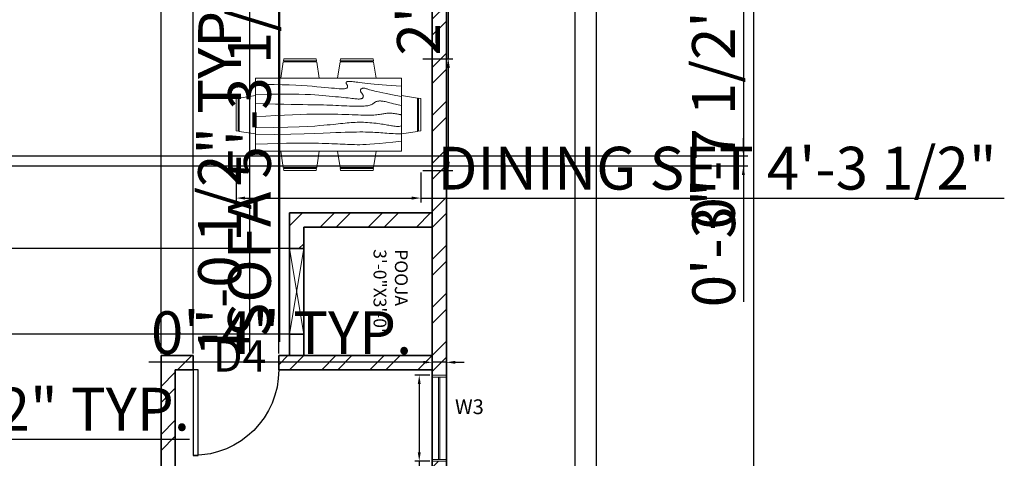
# Model space of a CAD drawing. Units: inches. Extents: x 2242 to 2870, y 1782 to 2635.
# Tile 4 of 7: x 2594 to 2870, y 2020 to 2143. Entities that reach past the tile are written whole.
import ezdxf

# ---------------------------------------------------------------- set-up
doc = ezdxf.new("R2010")
doc.units = ezdxf.units.IN
for name, color, linetype, lineweight in [('A-ANNO-DIMS', 7, 'Continuous', 18), ('A-ANNO-TEXT', 1, 'Continuous', 18), ('A-AREA-IDEN', 1, 'Continuous', 25), ('A-WALL-PATT', 253, 'Continuous', 13), ('C-PROP', 7, 'Continuous', 30), ('doors', 5, 'Continuous', 25), ('furniture', 9, 'Continuous', 18), ('walls', 7, 'Continuous', 35), ('windows', 72, 'Continuous', 18)]:
    doc.layers.add(name, color=color, linetype=linetype, lineweight=lineweight)
doc.styles.get("Standard").update_dxf_attribs({"font": 'arial.ttf'})
doc.dimstyles.new('ISO-25', dxfattribs={"dimtxt": 12, "dimasz": 2.5, "dimexe": 1.25, "dimexo": 0.625, "dimtad": 1, "dimlunit": 4, "dimtxsty": 'Standard', "dimcen": 2.5, "dimadec": 0, "dimazin": 0, "dimtfac": 1, "dimtmove": 0, "dimatfit": 3, "dimfxl": 1, "dimarcsym": 0})

# ---------------------------------------------------------------- blocks, each defined once
blk = doc.blocks.new('*U2')
for p, q in [((0, 0), (0, -5)), ((30, 0), (30, -5))]:
    blk.add_line(p, q)
blk.add_lwpolyline([(0, 0), (0, 30), (1.75, 30), (1.75, 0)], close=True)
blk.add_arc((0, 0), 30, 0, 90)
blk = doc.blocks.new('Dining Set - 36 x 72 in.')
for p, q in [((-22.2343, 26.00059), (-23.4847, 17.99762)), ((-22.2304, 26), (-5.7608, 26)), ((-22, 27.5), (-22.1562, 26.50042)), ((-5.8416, 26.5), (-22.1534, 26.5)), ((-22, 27.5), (-6, 27.5)), ((-5.8437, 26.49966), (-6, 27.5)), ((-4.5152, 17.99762), (-5.7655, 25.99926)), ((5.7657, 26.00059), (4.5153, 17.99762)), ((5.7696, 26), (22.2392, 26)), ((6, 27.5), (5.8438, 26.50042)), ((22.1584, 26.5), (5.8466, 26.5)), ((6, 27.5), (22, 27.5)), ((22.1563, 26.49966), (22, 27.5)), ((23.4848, 17.99762), (22.2345, 25.99926)), ((36, 18), (-36, 18)), ((-36, 18), (-36, -18)), ((36, -18), (36, 18)), ((-45.5, 8), (-44.5004, 8.15617)), ((-45.5, 8), (-45.5, -8)), ((-44.5, -8.15843), (-44.5, 8.15338)), ((-44.0006, 8.23428), (-35.9976, 9.48474)), ((-44, 8.23041), (-44, -8.23915)), ((44.0006, 8.23428), (35.9976, 9.48474)), ((44, 8.23041), (44, -8.23915)), ((44.5, -8.15843), (44.5, 8.15338)), ((45.5, 8), (44.5005, 8.15617)), ((45.5, 8), (45.5, -8)), ((-44.4997, -8.15631), (-45.5, -8)), ((-35.9976, -9.48476), (-43.9993, -8.2345)), ((35.9976, -9.48476), (43.9993, -8.2345)), ((44.4997, -8.15631), (45.5, -8)), ((-36, -18), (36, -18)), ((-22.2343, -26.0006), (-23.4847, -17.99762)), ((-4.5152, -17.99762), (-5.7655, -25.99928)), ((5.7657, -26.0006), (4.5153, -17.99762)), ((23.4848, -17.99762), (22.2345, -25.99928)), ((-22.2304, -26), (-5.7608, -26)), ((-22, -27.5), (-22.1562, -26.50044)), ((-5.8416, -26.5), (-22.1534, -26.5)), ((-22, -27.5), (-6, -27.5)), ((-5.8437, -26.49967), (-6, -27.5)), ((5.7696, -26), (22.2392, -26)), ((6, -27.5), (5.8438, -26.50044)), ((22.1584, -26.5), (5.8466, -26.5)), ((6, -27.5), (22, -27.5)), ((22.1563, -26.49967), (22, -27.5))]:
    blk.add_line(p, q)
for points in [[(-36, 15), (-31.1772, 14.97754), (-26.8079, 14.91406), (-22.8538, 14.81543), (-19.276, 14.6875), (-16.0362, 14.53613), (-13.0957, 14.36718), (-10.4159, 14.18652), (-7.9583, 14), (-5.6904, 13.81315), (-3.6035, 13.63021), (-1.6954, 13.45508), (0.0365, 13.29166), (1.5945, 13.14388), (2.9811, 13.01562), (4.1988, 12.9108), (5.25, 12.83333), (6.1393, 12.78613), (6.8802, 12.76823), (7.4883, 12.77767), (7.9792, 12.8125), (8.3685, 12.87077), (8.6719, 12.95052), (8.9049, 13.0498), (9.0833, 13.16666), (9.2205, 13.29899), (9.3216, 13.44401), (9.3895, 13.59879), (9.4271, 13.76041), (9.4373, 13.92594), (9.4232, 14.09245), (9.3875, 14.257), (9.3333, 14.41666), (9.2638, 14.56917), (9.1836, 14.71484), (9.0975, 14.85465), (9.0104, 14.98958), (8.9272, 15.1206), (8.8529, 15.2487), (8.7922, 15.37483), (8.75, 15.5), (8.7305, 15.62467), (8.7344, 15.74739), (8.7617, 15.86621), (8.8125, 15.97916), (8.8867, 16.08431), (8.9844, 16.17968), (9.1055, 16.26334), (9.25, 16.33333), (9.4189, 16.38802), (9.6172, 16.42708), (9.8506, 16.45052), (10.125, 16.45833), (10.4463, 16.45052), (10.8203, 16.42708), (11.2529, 16.38802), (11.75, 16.33333), (12.3184, 16.26318), (12.9694, 16.17838), (13.7151, 16.07991), (14.5677, 15.96875), (15.5395, 15.84586), (16.6426, 15.71224), (17.8893, 15.56884), (19.2917, 15.41666), (20.859, 15.25667), (22.5879, 15.08984), (24.4721, 14.91715), (26.5052, 14.73958), (28.6809, 14.5581), (30.9929, 14.3737), (33.4347, 14.18733), (36, 14)], [(-36, 10), (-28.9766, 10.14274), (-23.1725, 10.20442), (-18.4241, 10.19775), (-14.5677, 10.13541), (-11.4399, 10.03011), (-8.877, 9.89453), (-6.7154, 9.74137), (-4.7917, 9.58333), (-2.9698, 9.43082), (-1.2246, 9.28515), (0.4415, 9.14534), (2.026, 9.01041), (3.5266, 8.87939), (4.9408, 8.7513), (6.266, 8.62516), (7.5, 8.5), (8.6411, 8.37549), (9.6914, 8.2539), (10.6538, 8.13818), (11.5312, 8.03125), (12.3267, 7.93603), (13.043, 7.85547), (13.6831, 7.79248), (14.25, 7.75), (14.7471, 7.7303), (15.1797, 7.73307), (15.5537, 7.75732), (15.875, 7.80208), (16.1494, 7.86637), (16.3828, 7.94922), (16.5811, 8.04964), (16.75, 8.16666), (16.8944, 8.29915), (17.0143, 8.44531), (17.1089, 8.60319), (17.1771, 8.77083), (17.218, 8.94629), (17.2305, 9.1276), (17.2137, 9.31282), (17.1667, 9.5), (17.0895, 9.6875), (16.987, 9.875), (16.8649, 10.0625), (16.7292, 10.25), (16.5856, 10.4375), (16.4401, 10.625), (16.2985, 10.8125), (16.1667, 11), (16.05, 11.18733), (15.9518, 11.3737), (15.8752, 11.5581), (15.8229, 11.73958), (15.798, 11.91715), (15.8034, 12.08984), (15.842, 12.25667), (15.9167, 12.41666), (16.0295, 12.56836), (16.1784, 12.70833), (16.3605, 12.83268), (16.5729, 12.9375), (16.8127, 13.01888), (17.0768, 13.07291), (17.3625, 13.0957), (17.6667, 13.08333), (17.9894, 13.03312), (18.3418, 12.94726), (18.7382, 12.82918), (19.1927, 12.68229), (19.7195, 12.51001), (20.3327, 12.31575), (21.0465, 12.10294), (21.875, 11.875), (22.8357, 11.63354), (23.959, 11.37304), (25.2786, 11.08618), (26.8282, 10.76562), (28.6414, 10.40405), (30.752, 9.99414), (33.1936, 9.52856), (36, 9)], [(-36, 5.5), (-30.7157, 5.3348), (-26.069, 5.20963), (-21.9946, 5.11767), (-18.4271, 5.05208), (-15.3009, 5.00602), (-12.5508, 4.97265), (-10.1112, 4.94515), (-7.9167, 4.91666), (-5.909, 4.88167), (-4.0586, 4.83984), (-2.3429, 4.79215), (-0.7396, 4.73958), (0.7739, 4.6831), (2.22, 4.6237), (3.6213, 4.56233), (5, 4.5), (6.373, 4.43782), (7.7344, 4.3776), (9.0723, 4.32129), (10.375, 4.27083), (11.6309, 4.22819), (12.8281, 4.19531), (13.9551, 4.17415), (15, 4.16666), (15.954, 4.17448), (16.819, 4.19791), (17.6001, 4.23698), (18.3021, 4.29166), (18.9299, 4.36198), (19.4883, 4.44791), (19.9823, 4.54948), (20.4167, 4.66666), (20.7969, 4.79899), (21.1302, 4.94401), (21.4245, 5.09879), (21.6875, 5.26041), (21.9271, 5.42594), (22.1511, 5.59245), (22.3672, 5.757), (22.5834, 5.91666), (22.8065, 6.06868), (23.0404, 6.21093), (23.2879, 6.34147), (23.5521, 6.45833), (23.8358, 6.55957), (24.142, 6.64323), (24.4735, 6.70735), (24.8334, 6.75), (25.2235, 6.76969), (25.642, 6.76692), (26.0858, 6.74267), (26.5521, 6.69791), (27.0379, 6.63362), (27.5404, 6.55078), (28.0565, 6.45036), (28.5834, 6.33333), (29.1242, 6.19987), (29.7071, 6.04687), (30.3661, 5.87044), (31.1354, 5.66666), (32.0493, 5.43164), (33.142, 5.16146), (34.4475, 4.85221), (36, 4.5)], [(-36, -1), (-30.7915, -0.6591), (-26.0195, -0.38216), (-21.6519, -0.16284), (-17.6563, 0.00521), (-14.0005, 0.12833), (-10.6523, 0.21289), (-7.5796, 0.26522), (-4.75, 0.29166), (-2.134, 0.29793), (0.2878, 0.28711), (2.5317, 0.26163), (4.6146, 0.22396), (6.5529, 0.17651), (8.3633, 0.12174), (10.0623, 0.06209), (11.6667, 0), (13.1899, -0.06201), (14.6341, -0.1211), (15.9982, -0.17432), (17.2813, -0.21875), (18.4823, -0.25147), (19.6003, -0.26953), (20.6343, -0.27002), (21.5834, -0.25), (22.4481, -0.20768), (23.2357, -0.14584), (23.9549, -0.06836), (24.6146, 0.02083), (25.2235, 0.11784), (25.7904, 0.21875), (26.3241, 0.31966), (26.8334, 0.41666), (27.3265, 0.50618), (27.8099, 0.58593), (28.2894, 0.65397), (28.7709, 0.70833), (29.2601, 0.74707), (29.763, 0.76823), (30.2855, 0.76985), (30.8334, 0.75), (31.4088, 0.70784), (31.9994, 0.64713), (32.589, 0.57275), (33.1615, 0.48958), (33.7008, 0.4025), (34.1908, 0.3164), (34.6153, 0.23616), (34.9584, 0.16666), (35.2099, 0.11165), (35.3848, 0.07031), (35.504, 0.04069), (35.5886, 0.02083), (35.6594, 0.00879), (35.7377, 0.0026), (35.8442, 0.00032), (36, 0)], [(-36, -6.5), (-27.1843, -6.31267), (-20.084, -6.1263), (-14.469, -5.9419), (-10.1094, -5.76042), (-6.7752, -5.58285), (-4.2363, -5.41016), (-2.2629, -5.24333), (-0.625, -5.08334), (0.8708, -4.93099), (2.2715, -4.78646), (3.5872, -4.64974), (4.8281, -4.52084), (6.0046, -4.39974), (7.127, -4.28646), (8.2053, -4.18099), (9.25, -4.08334), (10.2705, -3.99382), (11.2734, -3.91407), (12.2647, -3.84603), (13.25, -3.79167), (14.2354, -3.75293), (15.2266, -3.73177), (16.2295, -3.73015), (17.25, -3.75), (18.2912, -3.79248), (19.3451, -3.85547), (20.4009, -3.93604), (21.4479, -4.03125), (22.4754, -4.13819), (23.4727, -4.25391), (24.4289, -4.37549), (25.3334, -4.5), (26.1785, -4.62492), (26.9694, -4.74935), (27.7145, -4.87281), (28.4219, -4.99479), (29.1, -5.11483), (29.7572, -5.23242), (30.4016, -5.34709), (31.0417, -5.45834), (31.6837, -5.56437), (32.3262, -5.65821), (32.9658, -5.73153), (33.599, -5.77604), (34.2224, -5.78345), (34.8327, -5.74545), (35.4264, -5.65373), (36, -5.5)], [(-36, -10), (-26.4022, -9.81299), (-18.4675, -9.62891), (-11.9839, -9.45069), (-6.7396, -9.28125), (-2.5226, -9.12354), (0.8789, -8.98047), (3.6769, -8.85498), (6.0833, -8.75), (8.2767, -8.66765), (10.3021, -8.60677), (12.1712, -8.56543), (13.8958, -8.54167), (15.4876, -8.53353), (16.9583, -8.53907), (18.3197, -8.55632), (19.5834, -8.58334), (20.7616, -8.61841), (21.8685, -8.66081), (22.9188, -8.71004), (23.9271, -8.76563), (24.9081, -8.82707), (25.8763, -8.89388), (26.8465, -8.96558), (27.8334, -9.04167), (28.8474, -9.12118), (29.8828, -9.20117), (30.93, -9.27824), (31.9792, -9.34896), (33.0205, -9.40991), (34.0443, -9.45768), (35.0407, -9.48885), (36, -9.5)], [(-36, -14.5), (-30.0881, -14.33513), (-25.0332, -14.21224), (-20.7312, -14.12647), (-17.0781, -14.07292), (-13.97, -14.04671), (-11.3027, -14.04297), (-8.9724, -14.05681), (-6.875, -14.08334), (-4.9224, -14.11833), (-3.0905, -14.16016), (-1.3709, -14.20785), (0.2448, -14.26042), (1.7647, -14.3169), (3.1973, -14.3763), (4.5507, -14.43767), (5.8333, -14.5), (7.0554, -14.5621), (8.235, -14.62175), (9.3922, -14.67652), (10.5469, -14.72396), (11.7192, -14.76164), (12.929, -14.78711), (14.1965, -14.79794), (15.5417, -14.79167), (16.9933, -14.76424), (18.6152, -14.70508), (20.4804, -14.60197), (22.6615, -14.44271), (25.2312, -14.21509), (28.2624, -13.9069), (31.8277, -13.50594), (36, -13)]]:
    blk.add_lwpolyline(points)
blk = doc.blocks.new('*D29')
at = {"layer": 'A-ANNO-DIMS', "color": 0, "lineweight": -2, "transparency": 16777216}
for p, q in [((2755.79, 2540.33), (2800.47, 2540.33)), ((2799.22, 2537.83), (2799.22, 1942.83)), ((2755.79, 1940.33), (2800.47, 1940.33))]:
    blk.add_line(p, q, dxfattribs=at)
at = {"layer": 'A-ANNO-DIMS', "color": 0, "transparency": 16777216}
for points in [[(2798.81, 2537.83), (2799.64, 2537.83), (2799.22, 2540.33)], [(2798.81, 1942.83), (2799.64, 1942.83), (2799.22, 1940.33)]]:
    blk.add_solid(points, dxfattribs=at)
at = {"layer": 'Defpoints', "color": 0, "transparency": 16777216}
for p in [(2755.16, 2540.33), (2755.16, 1940.33), (2799.22, 1940.33)]:
    blk.add_point(p, dxfattribs=at)
at = {"layer": 'A-ANNO-DIMS', "color": 0, "transparency": 16777216, "insert": (2792.47, 2240.33), "char_height": 12, "attachment_point": 5, "rotation": 90}
blk.add_mtext("50'", dxfattribs=at)
blk = doc.blocks.new('WIN-W3-24IN')
for p, q in [((0, 0), (0, 24.12)), ((0, 24.12), (4, 24.12)), ((0, 23.62), (4, 23.62)), ((1.8, 23.62), (1.8, 0.5)), ((2.2, 23.62), (2.2, 0.5)), ((4, 24.12), (4, 0)), ((4, 0.5), (0, 0.5)), ((4, 0), (0, 0))]:
    blk.add_line(p, q)
blk = doc.blocks.new('*D37')
at = {"layer": 'A-ANNO-DIMS', "color": 0, "lineweight": -2, "transparency": 16777216}
for p, q in [((2708.54, 2043.59), (2704.3, 2043.59)), ((2705.55, 2041.09), (2705.55, 2021.98)), ((2708.54, 2019.48), (2704.3, 2019.48)), ((2705.55, 2019.48), (2705.55, 1912.29))]:
    blk.add_line(p, q, dxfattribs=at)
at = {"layer": 'A-ANNO-DIMS', "color": 0, "transparency": 16777216}
for points in [[(2705.13, 2041.09), (2705.96, 2041.09), (2705.55, 2043.59)], [(2705.13, 2021.98), (2705.96, 2021.98), (2705.55, 2019.48)]]:
    blk.add_solid(points, dxfattribs=at)
at = {"layer": 'Defpoints', "color": 0, "transparency": 16777216}
for p in [(2709.16, 2043.59), (2705.55, 2019.48), (2709.16, 2019.48)]:
    blk.add_point(p, dxfattribs=at)
at = {"layer": 'A-ANNO-DIMS', "color": 0, "transparency": 16777216, "insert": (2698.79, 1964.63), "char_height": 12, "attachment_point": 5, "rotation": 90}
blk.add_mtext('W3 2\'-0" TYP.', dxfattribs=at)
blk = doc.blocks.new('*D38')
at = {"layer": 'A-ANNO-DIMS', "color": 0, "lineweight": -2, "transparency": 16777216}
for p, q in [((2709.16, 2044.22), (2709.16, 2048.46)), ((2713.16, 2044.22), (2713.16, 2048.46)), ((2706.66, 2047.21), (2629.77, 2047.21)), ((2713.16, 2047.21), (2709.16, 2047.21)), ((2715.66, 2047.21), (2718.16, 2047.21))]:
    blk.add_line(p, q, dxfattribs=at)
at = {"layer": 'A-ANNO-DIMS', "color": 0, "transparency": 16777216}
for points in [[(2706.66, 2047.63), (2706.66, 2046.79), (2709.16, 2047.21)], [(2715.66, 2047.63), (2715.66, 2046.79), (2713.16, 2047.21)]]:
    blk.add_solid(points, dxfattribs=at)
at = {"layer": 'Defpoints', "color": 0, "transparency": 16777216}
for p in [(2709.16, 2047.21), (2709.16, 2043.59), (2713.16, 2043.59)]:
    blk.add_point(p, dxfattribs=at)
at = {"layer": 'A-ANNO-DIMS', "color": 0, "transparency": 16777216, "insert": (2666.97, 2053.96), "char_height": 12, "attachment_point": 5}
blk.add_mtext('0\'-4" TYP.', dxfattribs=at)
blk = doc.blocks.new('*D42')
at = {"layer": 'A-ANNO-DIMS', "color": 0, "lineweight": -2, "transparency": 16777216}
for p, q in [((2522.93, 2020.21), (2522.93, 2026.94)), ((2537.42, 2020.21), (2537.42, 2026.94)), ((2525.43, 2025.69), (2534.92, 2025.69)), ((2537.42, 2025.69), (2641.15, 2025.69))]:
    blk.add_line(p, q, dxfattribs=at)
at = {"layer": 'A-ANNO-DIMS', "color": 0, "transparency": 16777216}
for points in [[(2525.43, 2026.11), (2525.43, 2025.28), (2522.93, 2025.69)], [(2534.92, 2026.11), (2534.92, 2025.28), (2537.42, 2025.69)]]:
    blk.add_solid(points, dxfattribs=at)
at = {"layer": 'Defpoints', "color": 0, "transparency": 16777216}
for p in [(2537.42, 2025.69), (2522.93, 2019.58), (2537.42, 2019.58)]:
    blk.add_point(p, dxfattribs=at)
at = {"layer": 'A-ANNO-DIMS', "color": 0, "transparency": 16777216, "insert": (2590.54, 2032.52), "char_height": 12, "attachment_point": 5}
blk.add_mtext('1\'-2 1/2" TYP.', dxfattribs=at)
blk = doc.blocks.new('*D44')
at = {"layer": 'A-ANNO-DIMS', "color": 0, "lineweight": -2, "transparency": 16777216}
for p, q in [((2659.56, 2164.94), (2656.71, 2164.94)), ((2657.96, 2162.44), (2657.96, 2155.17)), ((2659.56, 2152.67), (2656.71, 2152.67)), ((2657.96, 2152.67), (2657.96, 2048.94))]:
    blk.add_line(p, q, dxfattribs=at)
at = {"layer": 'A-ANNO-DIMS', "color": 0, "transparency": 16777216}
for points in [[(2657.54, 2162.44), (2658.38, 2162.44), (2657.96, 2164.94)], [(2657.54, 2155.17), (2658.38, 2155.17), (2657.96, 2152.67)]]:
    blk.add_solid(points, dxfattribs=at)
at = {"layer": 'Defpoints', "color": 0, "transparency": 16777216}
for p in [(2660.19, 2164.94), (2657.96, 2152.67), (2660.19, 2152.67)]:
    blk.add_point(p, dxfattribs=at)
at = {"layer": 'A-ANNO-DIMS', "color": 0, "transparency": 16777216, "insert": (2651.13, 2099.56), "char_height": 12, "attachment_point": 5, "rotation": 90}
blk.add_mtext('1\'-0 1/2" TYP.', dxfattribs=at)
blk = doc.blocks.new('*D51')
at = {"layer": 'A-ANNO-DIMS', "color": 0, "lineweight": -2, "transparency": 16777216}
for p, q in [((2654.22, 2100.4), (2654.22, 2092.02)), ((2705.95, 2100.4), (2705.95, 2092.02)), ((2656.72, 2093.27), (2703.45, 2093.27)), ((2705.95, 2093.27), (2869.55, 2093.27))]:
    blk.add_line(p, q, dxfattribs=at)
at = {"layer": 'A-ANNO-DIMS', "color": 0, "transparency": 16777216}
for points in [[(2656.72, 2093.69), (2656.72, 2092.85), (2654.22, 2093.27)], [(2703.45, 2093.69), (2703.45, 2092.85), (2705.95, 2093.27)]]:
    blk.add_solid(points, dxfattribs=at)
at = {"layer": 'Defpoints', "color": 0, "transparency": 16777216}
for p in [(2654.22, 2101.03), (2705.95, 2101.03), (2705.95, 2093.27)]:
    blk.add_point(p, dxfattribs=at)
at = {"layer": 'A-ANNO-DIMS', "color": 0, "transparency": 16777216, "insert": (2789, 2100.1), "char_height": 12, "attachment_point": 5}
blk.add_mtext('DINING SET 4\'-3 1/2"', dxfattribs=at)
blk = doc.blocks.new('*D52')
at = {"layer": 'A-ANNO-DIMS', "color": 0, "lineweight": -2, "transparency": 16777216}
for p, q in [((2713.71, 2132.29), (2713.71, 2196.1)), ((2706.57, 2132.29), (2714.96, 2132.29)), ((2713.71, 2103.53), (2713.71, 2129.79)), ((2706.57, 2101.03), (2714.96, 2101.03))]:
    blk.add_line(p, q, dxfattribs=at)
at = {"layer": 'A-ANNO-DIMS', "color": 0, "transparency": 16777216}
for points in [[(2713.29, 2129.79), (2714.12, 2129.79), (2713.71, 2132.29)], [(2713.29, 2103.53), (2714.12, 2103.53), (2713.71, 2101.03)]]:
    blk.add_solid(points, dxfattribs=at)
at = {"layer": 'Defpoints', "color": 0, "transparency": 16777216}
for p in [(2705.95, 2132.29), (2713.71, 2132.29), (2705.95, 2101.03)]:
    blk.add_point(p, dxfattribs=at)
at = {"layer": 'A-ANNO-DIMS', "color": 0, "transparency": 16777216, "insert": (2706.88, 2165.45), "char_height": 12, "attachment_point": 5, "rotation": 90}
blk.add_mtext('2\'-7 1/2"', dxfattribs=at)
blk = doc.blocks.new('*D53')
at = {"layer": 'A-ANNO-DIMS', "color": 0, "lineweight": -2, "transparency": 16777216}
for p, q in [((2675.25, 2230.42), (2665.09, 2230.42)), ((2666.34, 2227.92), (2666.34, 2169.35)), ((2675.25, 2166.85), (2665.09, 2166.85)), ((2666.34, 2166.85), (2666.34, 2053))]:
    blk.add_line(p, q, dxfattribs=at)
at = {"layer": 'A-ANNO-DIMS', "color": 0, "transparency": 16777216}
for points in [[(2665.92, 2227.92), (2666.76, 2227.92), (2666.34, 2230.42)], [(2665.92, 2169.35), (2666.76, 2169.35), (2666.34, 2166.85)]]:
    blk.add_solid(points, dxfattribs=at)
at = {"layer": 'Defpoints', "color": 0, "transparency": 16777216}
for p in [(2675.87, 2230.42), (2666.34, 2166.85), (2675.87, 2166.85)]:
    blk.add_point(p, dxfattribs=at)
at = {"layer": 'A-ANNO-DIMS', "color": 0, "transparency": 16777216, "insert": (2659.5, 2108.68), "char_height": 12, "attachment_point": 5, "rotation": 90}
blk.add_mtext('SOFA 5\'-3 1/2"', dxfattribs=at)
blk = doc.blocks.new('*D64')
at = {"layer": 'A-ANNO-DIMS', "color": 0, "lineweight": -2, "transparency": 16777216}
for p, q in [((2642.16, 2049.72), (2642.16, 2611.83)), ((2666.16, 2049.72), (2666.16, 2611.83)), ((2644.66, 2610.58), (2663.66, 2610.58)), ((2666.16, 2610.58), (2702.02, 2610.58))]:
    blk.add_line(p, q, dxfattribs=at)
at = {"layer": 'A-ANNO-DIMS', "color": 0, "transparency": 16777216}
for points in [[(2644.66, 2611), (2644.66, 2610.17), (2642.16, 2610.58)], [(2663.66, 2611), (2663.66, 2610.17), (2666.16, 2610.58)]]:
    blk.add_solid(points, dxfattribs=at)
at = {"layer": 'Defpoints', "color": 0, "transparency": 16777216}
for p in [(2666.16, 2610.58), (2642.16, 2049.1), (2666.16, 2049.1)]:
    blk.add_point(p, dxfattribs=at)
at = {"layer": 'A-ANNO-DIMS', "color": 0, "transparency": 16777216, "insert": (2685.34, 2617.34), "char_height": 12, "attachment_point": 5}
blk.add_mtext('2\'-0"', dxfattribs=at)
blk = doc.blocks.new('*D77')
at = {"layer": 'A-ANNO-DIMS', "color": 0, "lineweight": -2, "transparency": 16777216}
for p, q in [((2393.37, 2157.1), (2797.66, 2157.1)), ((2796.41, 2154.6), (2796.41, 2152.19)), ((2393.37, 2149.69), (2797.66, 2149.69)), ((2796.41, 2149.69), (2796.41, 2086.08))]:
    blk.add_line(p, q, dxfattribs=at)
at = {"layer": 'A-ANNO-DIMS', "color": 0, "transparency": 16777216}
for points in [[(2796, 2154.6), (2796.83, 2154.6), (2796.41, 2157.1)], [(2796, 2152.19), (2796.83, 2152.19), (2796.41, 2149.69)]]:
    blk.add_solid(points, dxfattribs=at)
at = {"layer": 'Defpoints', "color": 0, "transparency": 16777216}
for p in [(2392.74, 2157.1), (2392.74, 2149.69), (2796.41, 2149.69)]:
    blk.add_point(p, dxfattribs=at)
at = {"layer": 'A-ANNO-DIMS', "color": 0, "transparency": 16777216, "insert": (2789.58, 2116.64), "char_height": 12, "attachment_point": 5, "rotation": 90}
blk.add_mtext('0\'-7 1/2"', dxfattribs=at)
blk = doc.blocks.new('*D78')
at = {"layer": 'A-ANNO-DIMS', "color": 0, "lineweight": -2, "transparency": 16777216}
for p, q in [((2796.41, 2107.6), (2796.41, 2110.1)), ((2393.37, 2105.1), (2797.66, 2105.1)), ((2796.41, 2105.1), (2796.41, 2102.29)), ((2393.37, 2102.29), (2797.66, 2102.29)), ((2796.41, 2099.79), (2796.41, 2064.14))]:
    blk.add_line(p, q, dxfattribs=at)
at = {"layer": 'A-ANNO-DIMS', "color": 0, "transparency": 16777216}
for points in [[(2796, 2107.6), (2796.83, 2107.6), (2796.41, 2105.1)], [(2796, 2099.79), (2796.83, 2099.79), (2796.41, 2102.29)]]:
    blk.add_solid(points, dxfattribs=at)
at = {"layer": 'Defpoints', "color": 0, "transparency": 16777216}
for p in [(2392.74, 2105.1), (2392.74, 2102.29), (2796.41, 2102.29)]:
    blk.add_point(p, dxfattribs=at)
at = {"layer": 'A-ANNO-DIMS', "color": 0, "transparency": 16777216, "insert": (2789.66, 2080.72), "char_height": 12, "attachment_point": 5, "rotation": 90}
blk.add_mtext('0\'-3"', dxfattribs=at)
blk = doc.blocks.new('*D81')
at = {"layer": 'A-ANNO-DIMS', "color": 0, "lineweight": -2, "transparency": 16777216}
for p, q in [((2266.89, 2079.1), (2266.89, 2114.95)), ((2672.54, 2079.1), (2265.64, 2079.1)), ((2266.89, 2057.6), (2266.89, 2076.6)), ((2672.54, 2055.1), (2265.64, 2055.1))]:
    blk.add_line(p, q, dxfattribs=at)
at = {"layer": 'A-ANNO-DIMS', "color": 0, "transparency": 16777216}
for points in [[(2266.47, 2076.6), (2267.3, 2076.6), (2266.89, 2079.1)], [(2266.47, 2057.6), (2267.3, 2057.6), (2266.89, 2055.1)]]:
    blk.add_solid(points, dxfattribs=at)
at = {"layer": 'Defpoints', "color": 0, "transparency": 16777216}
for p in [(2266.89, 2079.1), (2673.16, 2079.1), (2673.16, 2055.1)]:
    blk.add_point(p, dxfattribs=at)
at = {"layer": 'A-ANNO-DIMS', "color": 0, "transparency": 16777216, "insert": (2260.13, 2098.27), "char_height": 12, "attachment_point": 5, "rotation": 90}
blk.add_mtext('2\'-0"', dxfattribs=at)
blk = doc.blocks.new('*D82')
at = {"layer": 'A-ANNO-DIMS', "color": 0, "lineweight": -2, "transparency": 16777216}
for p, q in [((2633.16, 2049.72), (2633.16, 2611.83)), ((2642.16, 2049.72), (2642.16, 2611.83)), ((2633.16, 2610.58), (2597.51, 2610.58)), ((2639.66, 2610.58), (2635.66, 2610.58))]:
    blk.add_line(p, q, dxfattribs=at)
at = {"layer": 'A-ANNO-DIMS', "color": 0, "transparency": 16777216}
for points in [[(2635.66, 2611), (2635.66, 2610.17), (2633.16, 2610.58)], [(2639.66, 2611), (2639.66, 2610.17), (2642.16, 2610.58)]]:
    blk.add_solid(points, dxfattribs=at)
at = {"layer": 'Defpoints', "color": 0, "transparency": 16777216}
for p in [(2633.16, 2610.58), (2633.16, 2049.1), (2642.16, 2049.1)]:
    blk.add_point(p, dxfattribs=at)
at = {"layer": 'A-ANNO-DIMS', "color": 0, "transparency": 16777216, "insert": (2614.09, 2617.34), "char_height": 12, "attachment_point": 5}
blk.add_mtext('0\'-9"', dxfattribs=at)

msp = doc.modelspace()

# ---------------------------------------------------------------- hatches: boundary and pattern name
at = {"layer": 'A-WALL-PATT'}
h = msp.add_hatch(dxfattribs=at)
h.set_pattern_fill('ANSI32', color=256)
h.paths.add_polyline_path([(2713.164, 2198.138), (2709.164, 2198.138), (2709.164, 2043.592), (2713.164, 2043.592)])
h = msp.add_hatch(dxfattribs=at)
h.set_pattern_fill('ANSI32', color=256)
h.paths.add_polyline_path([(2709.164, 2089.097), (2669.164, 2089.097), (2669.164, 2079.097), (2673.164, 2079.097), (2673.164, 2085.097), (2709.164, 2085.097)])
h = msp.add_hatch(dxfattribs=at)
h.set_pattern_fill('ANSI32', color=256)
h.paths.add_polyline_path([(2713.164, 2019.476), (2709.164, 2019.476), (2709.164, 1961.097), (2637.164, 1961.097), (2637.164, 2045.097), (2642.164, 2045.097), (2642.164, 2049.097), (2633.164, 2049.097), (2633.164, 1961.097), (2630.164, 1961.097), (2630.164, 1957.097), (2713.164, 1957.097)])
h = msp.add_hatch(dxfattribs=at)
h.set_pattern_fill('ANSI32', color=256)
h.paths.add_polyline_path([(2709.164, 2049.097), (2666.164, 2049.097), (2666.164, 2045.097), (2709.164, 2045.097)], flags=17)

# ---------------------------------------------------------------- linework, layer by layer
at = {"layer": 'C-PROP'}
for p, q in [((2755.164, 2540.335), (2755.164, 1940.335)), ((2749.164, 2534.335), (2749.164, 1945.097))]:
    msp.add_line(p, q, dxfattribs=at)
at = {"layer": 'walls'}
for p, q in [((2709.164, 2254.097), (2709.164, 1961.097)), ((2713.164, 2254.097), (2713.164, 1957.097)), ((2709.164, 2089.097), (2669.164, 2089.097)), ((2669.164, 2089.097), (2669.164, 2049.097)), ((2709.164, 2085.097), (2673.164, 2085.097)), ((2673.164, 2085.097), (2673.164, 2049.097)), ((2673.164, 2085.097), (2673.164, 2079.097)), ((2673.164, 2079.097), (2669.164, 2079.097)), ((2669.164, 2049.097), (2669.164, 2055.097)), ((2669.164, 2055.097), (2673.164, 2055.097)), ((2633.164, 2049.097), (2633.164, 1961.097)), ((2642.164, 2049.097), (2633.164, 2049.097)), ((2642.164, 2045.097), (2642.164, 2049.097)), ((2709.164, 2049.097), (2666.164, 2049.097)), ((2669.164, 2049.097), (2666.164, 2049.097)), ((2666.164, 2049.097), (2666.164, 2045.097)), ((2637.164, 2045.097), (2637.164, 1961.097)), ((2642.164, 2045.097), (2637.164, 2045.097)), ((2709.164, 2045.097), (2666.164, 2045.097))]:
    msp.add_line(p, q, dxfattribs=at)
at = {"layer": 'windows'}
for p, q in [((2673.164, 2079.097), (2669.164, 2055.097)), ((2669.164, 2079.097), (2673.164, 2055.097))]:
    msp.add_line(p, q, dxfattribs=at)

# ---------------------------------------------------------------- block references
at = {"layer": 'doors', "xscale": -0.8, "yscale": 0.8, "zscale": 0.8, "rotation": 180}
msp.add_blockref('*U2', (2642.164, 2045.097), dxfattribs=at)
at = {"layer": 'furniture', "xscale": 0.5683868703205625, "yscale": 0.5683868703205625, "zscale": 0.5683868703205625}
msp.add_blockref('Dining Set - 36 x 72 in.', (2680.086, 2116.658), dxfattribs=at)
at = {"layer": 'windows', "rotation": 180}
msp.add_blockref('WIN-W3-24IN', (2713.163, 2043.592), dxfattribs=at)

# ---------------------------------------------------------------- texts
at = {"layer": 'A-ANNO-TEXT', "attachment_point": 1}
for s, width, gutter_width, insert, char_height in [('D4', 1.59204, 9.179, (2647.762, 2053.414), 8.8122), ('W3', 1.14454, 20.658, (2715.573, 2036.818), 4.1316)]:
    msp.add_mtext_dynamic_manual_height_columns(s, width=width, gutter_width=gutter_width, heights=[0], dxfattribs=dict(at, insert=insert, char_height=char_height))
at = {"layer": 'A-AREA-IDEN', "insert": (2702.298, 2078.918), "char_height": 3.58088, "attachment_point": 1, "rotation": 270}
msp.add_mtext_dynamic_manual_height_columns('POOJA\\P3\'-0"X3\'-0"', width=0.38333, gutter_width=17.904, heights=[0], dxfattribs=at)

# ---------------------------------------------------------------- dimensions: what is measured, and where the dimension line sits
at = {"layer": 'A-ANNO-DIMS'}
for base, p2, picture, middle in [((2633.164, 2610.585), (2633.164, 2049.097), '*D82', (2614.089, 2617.337)), ((2666.164, 2610.585), (2666.164, 2049.097), '*D64', (2685.34, 2617.337))]:
    dim = msp.add_linear_dim(base=base, p1=(2642.164, 2049.097), p2=p2, dimstyle='ISO-25', override={"dimdec": 1, "dimlfac": 1, "dimrnd": 0, "dimzin": 1, "dimdsep": 46, "dimlunit": 4, "dimfrac": 2}, dxfattribs=at)
    dim.commit()
    dim.dimension.update_dxf_attribs({"geometry": picture, "text_midpoint": middle})
for base, p1, p2, override, picture, middle in [((2799.223, 1940.335), (2755.164, 2540.335), (2755.164, 1940.335), {"dimclrd": 0, "dimclre": 0, "dimclrt": 0}, '*D29', (2792.471, 2240.335)), ((2713.706, 2132.289), (2705.947, 2101.027), (2705.947, 2132.289), {"dimdec": 1, "dimlfac": 1, "dimrnd": 0, "dimzin": 1, "dimdsep": 46, "dimlunit": 4, "dimfrac": 2}, '*D52', (2706.876, 2165.446)), ((2796.414, 2149.693), (2392.745, 2157.097), (2392.745, 2149.693), {"dimdec": 1, "dimlfac": 1, "dimrnd": 0, "dimzin": 1, "dimdsep": 46, "dimlunit": 4, "dimfrac": 2}, '*D77', (2789.584, 2116.638)), ((2266.887, 2079.097), (2673.164, 2055.097), (2673.164, 2079.097), {"dimdec": 1, "dimlfac": 1, "dimrnd": 0, "dimzin": 1, "dimdsep": 46, "dimlunit": 4, "dimfrac": 2}, '*D81', (2260.135, 2098.274)), ((2796.414, 2102.29), (2392.745, 2105.097), (2392.745, 2102.29), {"dimdec": 1, "dimlfac": 1, "dimrnd": 0, "dimzin": 1, "dimdsep": 46, "dimlunit": 4, "dimfrac": 2}, '*D78', (2789.658, 2080.716))]:
    dim = msp.add_linear_dim(base=base, p1=p1, p2=p2, angle=90, dimstyle='ISO-25', override=override, dxfattribs=at)
    dim.commit()
    dim.dimension.update_dxf_attribs({"geometry": picture, "text_midpoint": middle})
for base, p1, p2, angle, text, picture, middle in [((2666.339, 2166.855), (2675.874, 2230.422), (2675.874, 2166.855), 270, 'SOFA <>', '*D53', (2659.501, 2108.678)), ((2657.959, 2152.672), (2660.189, 2164.94), (2660.189, 2152.672), 270, '<> TYP.', '*D44', (2651.13, 2099.558)), ((2709.164, 2047.209), (2713.164, 2043.592), (2709.164, 2043.592), 180, '<> TYP.', '*D38', (2666.966, 2053.961)), ((2705.546, 2019.476), (2709.164, 2043.592), (2709.164, 2019.476), 270, 'W3 <> TYP.', '*D37', (2698.79, 1964.631))]:
    dim = msp.add_linear_dim(base=base, p1=p1, p2=p2, angle=angle, text=text, dimstyle='ISO-25', override={"dimdec": 1, "dimlfac": 1, "dimrnd": 0, "dimzin": 1, "dimdsep": 46, "dimlunit": 4, "dimfrac": 2}, dxfattribs=at)
    dim.commit()
    dim.dimension.update_dxf_attribs({"geometry": picture, "text_midpoint": middle})
for base, p1, p2, text, picture, middle in [((2705.947, 2093.269), (2654.224, 2101.027), (2705.947, 2101.027), 'DINING SET <>', '*D51', (2789, 2100.103)), ((2537.424, 2025.694), (2522.931, 2019.58), (2537.424, 2019.58), '<> TYP.', '*D42', (2590.538, 2032.524))]:
    dim = msp.add_linear_dim(base=base, p1=p1, p2=p2, text=text, dimstyle='ISO-25', override={"dimdec": 1, "dimlfac": 1, "dimrnd": 0, "dimzin": 1, "dimdsep": 46, "dimlunit": 4, "dimfrac": 2}, dxfattribs=at)
    dim.commit()
    dim.dimension.update_dxf_attribs({"geometry": picture, "text_midpoint": middle})

doc.saveas('drawing.dxf')
